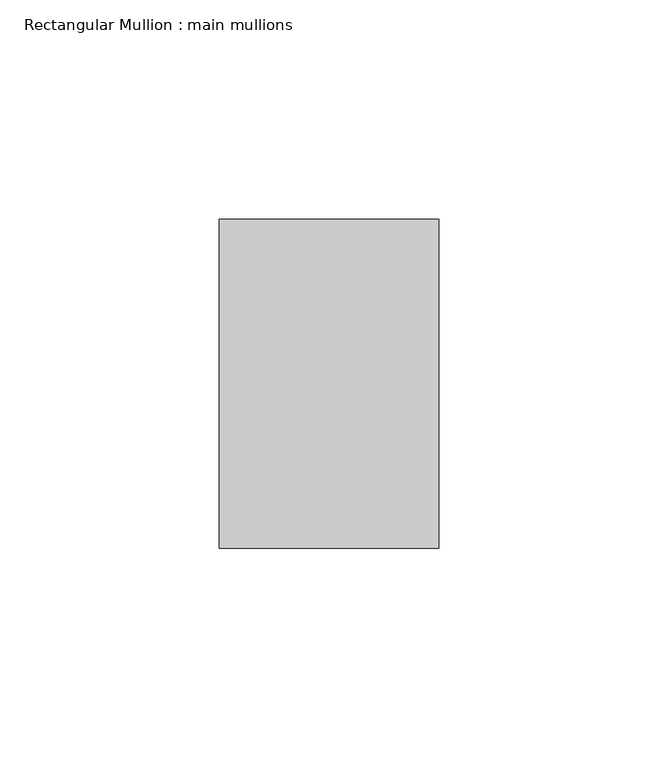
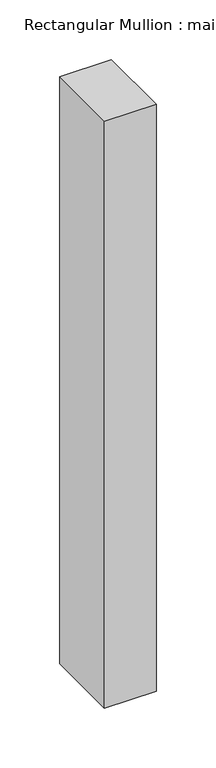
"""IFC4 building model written with IfcOpenShell, lengths in millimetres: member geometry, Rectangular Mullion : main mullions."""

from ifc_helpers import new_model, si_unit, frame, origin, place, context, project, spatial, polyline, outline, extrude, source, transform, mapped, element, save


def rectangular_mullion_main_mullions_6d09e4bf(model_context):
    return source(origin(), model_context, "Body", "SweptSolid", [
        extrude(outline(polyline([(25.0, 37.5), (25.0, -37.5), (-25.0, -37.5), (-25.0, 37.5), (25.0, 37.5)])), frame((0.0, 0.0, -600.0), z_axis=(0.0, 0.0, 1.0), x_axis=(1.0, 0.0, 0.0)), (0.0, 0.0, 1.0), 600.0),
    ])


if __name__ == "__main__":
    model = new_model("IFC4")
    model_context = context("Model", 3, world=origin())
    ifc_project = project(units=[si_unit("LENGTHUNIT", "METRE", prefix="MILLI")], contexts=[model_context])
    site = spatial("IfcSite", under=ifc_project)
    building = spatial("IfcBuilding", under=site)
    placement = place(None, origin())
    rectangular_mullion_main_mullions_shape = rectangular_mullion_main_mullions_6d09e4bf(model_context)
    element("IfcMember", 1, ObjectType="Rectangular Mullion : main mullions", at=placement, inside=building, context=model_context, shape_type="MappedRepresentation", body=[
        mapped(rectangular_mullion_main_mullions_shape, transform((0.0, 0.0, 0.0), x_axis=(1.0, 0.0, 0.0), y_axis=(0.0, 1.0, 0.0), z_axis=(0.0, 0.0, 1.0))),
    ])
    save(model, "model.ifc")

# Revit data of these elements
# Type "Rectangular Mullion : main mullions"
#   built-in parameter 1007304 = 0.246063 (stored number, unit not read)
#   built-in parameter 1007301 = 0.082021 (stored number, unit not read)
#   built-in parameter 1007300 = 0.082021 (stored number, unit not read)
# Element 1 (IfcMember, "Rectangular Mullion : main mullions")
#   Materials on its faces: "Aluminum"
# Materials
#   "Aluminum": class "Metal", colour RGB 136 136 136, transparency 0, Description = "Aluminum 6061", Cost = 0
